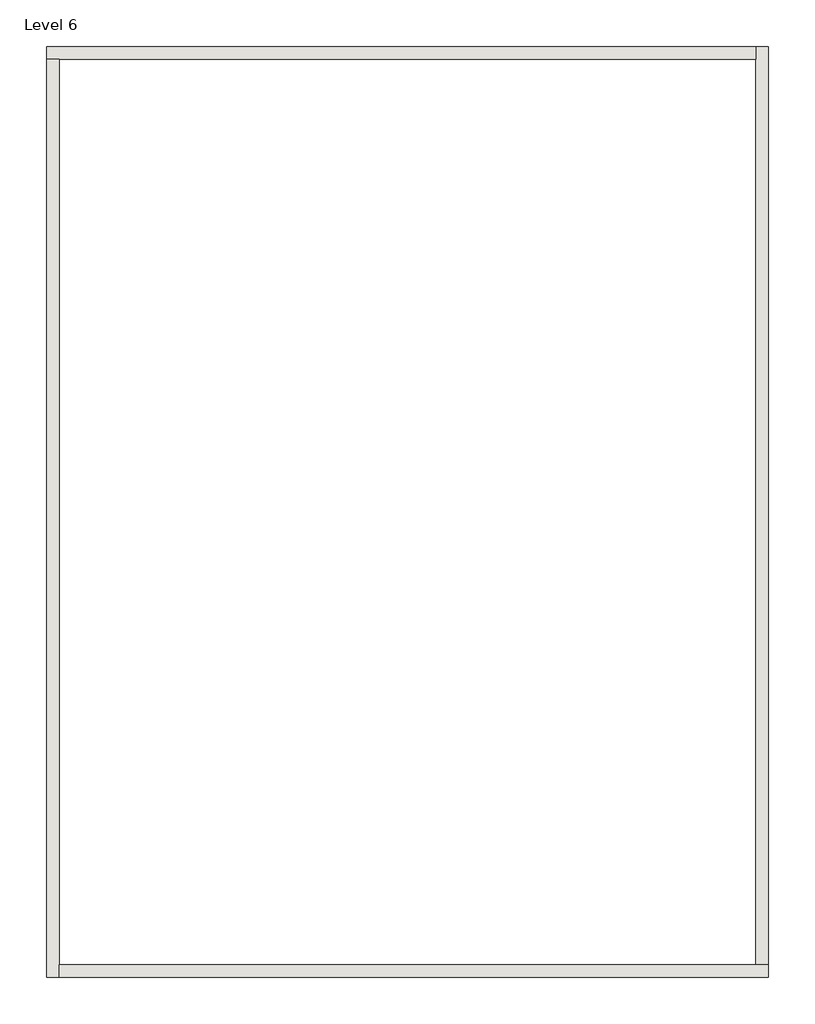
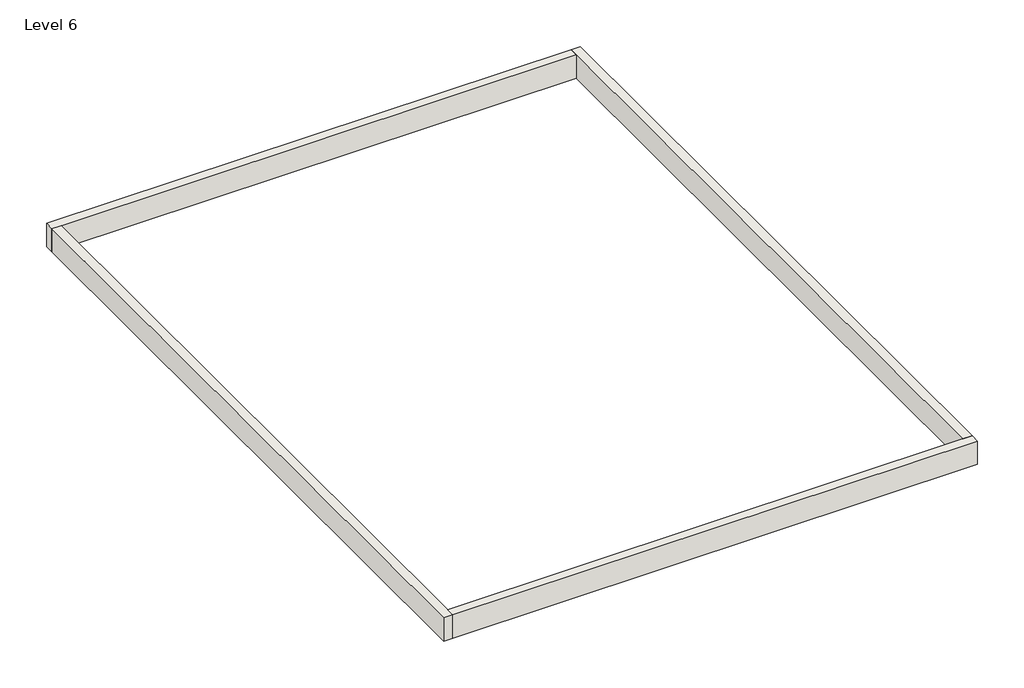
# One storey, incomplete: 4 walls.
"""IFC4 building model written with IfcOpenShell, lengths in millimetres."""

from ifc_helpers import new_model, si_unit, origin, place, context, project, spatial, faceted_brep, element, save

model = new_model("IFC4")

# Units and contexts
model_context = context("Model", 3, world=origin())
ifc_project = project(units=[si_unit("LENGTHUNIT", "METRE", prefix="MILLI")], contexts=[model_context])

# Site, building, storey
site = spatial("IfcSite", under=ifc_project)
building = spatial("IfcBuilding", under=site)
storey = spatial("IfcBuildingStorey", under=building, Name="Level 6", Elevation=15240.0)

# Walls
placement = place(None, origin())
element("IfcWall", 1, ObjectType="Generic - 4.5\"", at=placement, inside=storey, context=model_context, shape_type="Brep", body=[
    faceted_brep([(-7871.9415084, 8793.1935985, 15240.0), (-7643.3415084, 8793.1935985, 15240.0), (5082.0584916, 8793.1935985, 15240.0), (5082.0584916, 8793.1935985, 15849.6), (-7643.3415084, 8793.1935985, 15849.6), (-7871.9415084, 8793.1935985, 15849.6), (-7871.9415084, 9021.7935985, 15240.0), (-7871.9415084, 9021.7935985, 15849.6), (5082.0584916, 9021.7935985, 15849.6), (5082.0584916, 9021.7935985, 15240.0)], [[[0, 1, 2, 3, 4, 5]], [[6, 7, 8, 9]], [[2, 1, 0, 6, 9]], [[5, 4, 3, 8, 7]], [[0, 5, 7, 6]], [[3, 2, 9, 8]]]),
])
element("IfcWall", 2, ObjectType="Generic - 4.5\"", at=placement, inside=storey, context=model_context, shape_type="Brep", body=[
    faceted_brep([(-7643.3415084, -7970.8064015, 15240.0), (-7643.3415084, -7742.2064015, 15240.0), (-7643.3415084, 8793.1935985, 15240.0), (-7643.3415084, 8793.1935985, 15849.6), (-7643.3415084, -7742.2064015, 15849.6), (-7643.3415084, -7970.8064015, 15849.6), (-7871.9415084, -7970.8064015, 15240.0), (-7871.9415084, -7970.8064015, 15849.6), (-7871.9415084, 8793.1935985, 15849.6), (-7871.9415084, 8793.1935985, 15240.0)], [[[0, 1, 2, 3, 4, 5]], [[6, 7, 8, 9]], [[2, 1, 0, 6, 9]], [[5, 4, 3, 8, 7]], [[0, 5, 7, 6]], [[3, 2, 9, 8]]]),
])
element("IfcWall", 3, ObjectType="Generic - 4.5\"", at=placement, inside=storey, context=model_context, shape_type="Brep", body=[
    faceted_brep([(5310.6584916, -7742.2064015, 15240.0), (5082.0584916, -7742.2064015, 15240.0), (-7643.3415084, -7742.2064015, 15240.0), (-7643.3415084, -7742.2064015, 15849.6), (5082.0584916, -7742.2064015, 15849.6), (5310.6584916, -7742.2064015, 15849.6), (5310.6584916, -7970.8064015, 15240.0), (5310.6584916, -7970.8064015, 15849.6), (-7643.3415084, -7970.8064015, 15849.6), (-7643.3415084, -7970.8064015, 15240.0)], [[[0, 1, 2, 3, 4, 5]], [[6, 7, 8, 9]], [[2, 1, 0, 6, 9]], [[5, 4, 3, 8, 7]], [[0, 5, 7, 6]], [[3, 2, 9, 8]]]),
])
element("IfcWall", 4, ObjectType="Generic - 4.5\"", at=placement, inside=storey, context=model_context, shape_type="Brep", body=[
    faceted_brep([(5082.0584916, 9021.7935985, 15240.0), (5082.0584916, 8793.1935985, 15240.0), (5082.0584916, -7742.2064015, 15240.0), (5082.0584916, -7742.2064015, 15849.6), (5082.0584916, 8793.1935985, 15849.6), (5082.0584916, 9021.7935985, 15849.6), (5310.6584916, 9021.7935985, 15240.0), (5310.6584916, 9021.7935985, 15849.6), (5310.6584916, -7742.2064015, 15849.6), (5310.6584916, -7742.2064015, 15240.0)], [[[0, 1, 2, 3, 4, 5]], [[6, 7, 8, 9]], [[2, 1, 0, 6, 9]], [[5, 4, 3, 8, 7]], [[0, 5, 7, 6]], [[3, 2, 9, 8]]]),
])

save(model, "model.ifc")

# Revit data of these elements
# Type "Generic - 4.5\""
#   Assembly Code = "B2010"
#   Layers, outside or top first: 0' - 9" no material (function 1)
# Elements 1, 4 (IfcWall, "Generic - 4.5\"")
#   Top Offset = 0' - 0"
#   Base Offset = 0' - 0"
#   Unconnected Height = 2' - 0"
#   wall height = 2' - 0"
#   Phase Created = New Construction
#   Base Constraint = Level 6
#   Materials on its faces: "Default Wall", "Bed-white fabric"
# Element 2 (IfcWall, "Generic - 4.5\"")
#   Top Offset = 0' - 0"
#   Base Offset = 0' - 0"
#   Unconnected Height = 2' - 0"
#   wall height = 2' - 0"
#   Phase Created = New Construction
#   Base Constraint = Level 6
#   Materials on its faces: "Default Wall", "Bed-white fabric", "Default Mass Interior Wall"
# Element 3 (IfcWall, "Generic - 4.5\"")
#   Top Offset = 0' - 0"
#   Base Offset = 0' - 0"
#   Unconnected Height = 2' - 0"
#   wall height = 2' - 0"
#   Phase Created = New Construction
#   Base Constraint = Level 6
#   Materials on its faces: "Default Wall", "Default Mass Interior Wall", "Bed-white fabric"
# Materials
#   "Default Wall": colour RGB 128 128 128, transparency 0, Cost = 0
#   "Bed-white fabric": class "Paint", colour RGB 220 220 220, transparency 0
#   "Default Mass Interior Wall": class "Generic", colour RGB 195 229 126, transparency 0, Cost = 0
